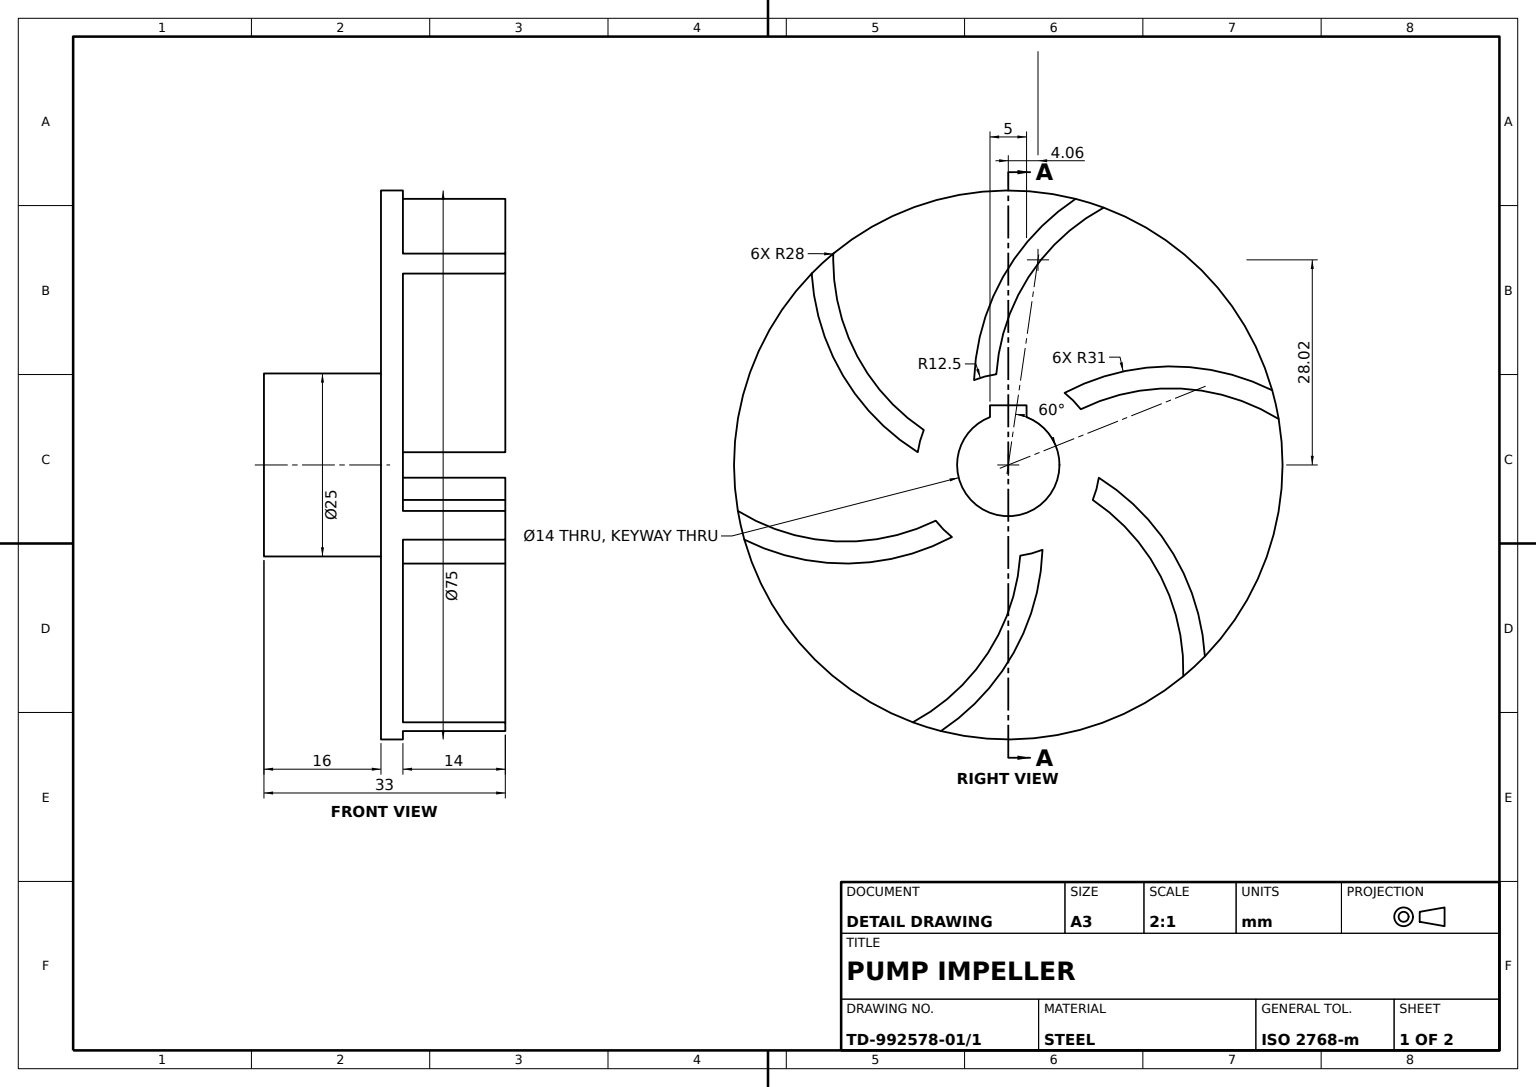
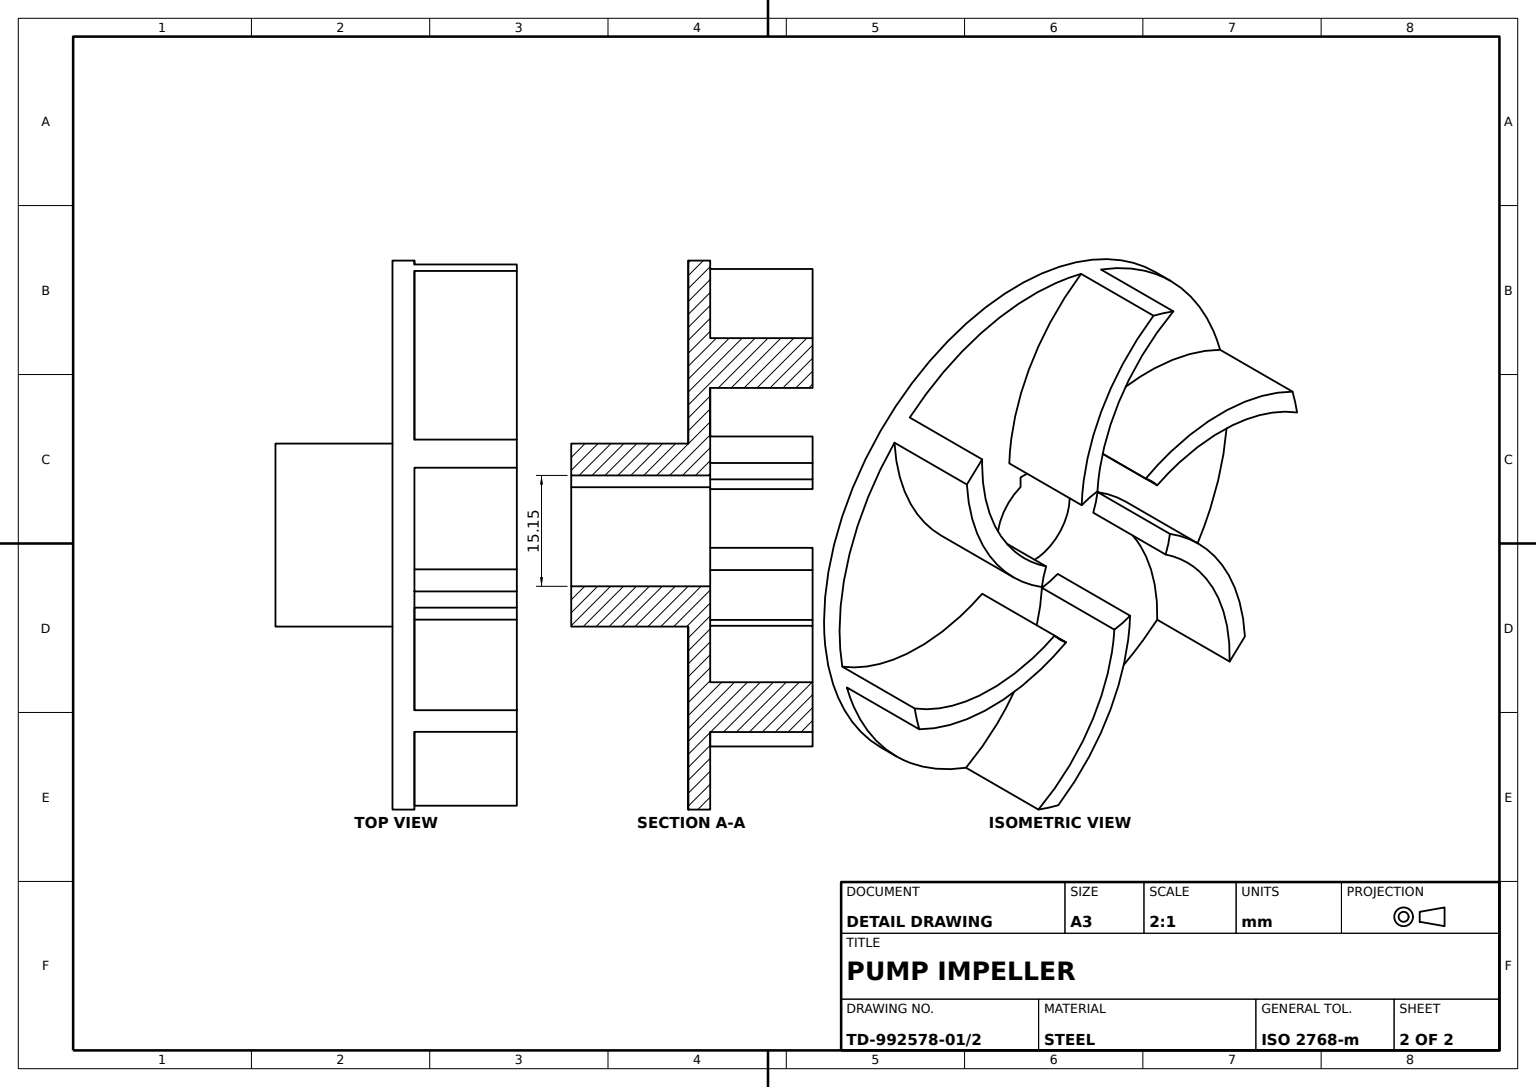
SolidWorks part; units mm, degrees
material "Plain Carbon Steel"
ref_plane "Front Plane" through (0, 0, 0) normal (0, 0, 1) x (1, 0, 0)
ref_plane "Top Plane" through (0, 0, 0) normal (0, 1, 0) x (1, 0, 0)
ref_plane "Right Plane" through (0, 0, 0) normal (1, 0, 0) x (0, 0, -1)
sketch "Hub Disc Profile" plane through (0, 0, 0) normal (0, 0, 1) x (1, 0, 0)
  line L0 (0, 12.5) -> (0, -20.8889) construction
  line L1 (-28, 0) -> (30.1111, 0) construction
  line L2 (0, 12.5) -> (0, 7)
  line L4 (0, 12.5) -> (16, 12.5)
  line L5 (16, 12.5) -> (16, 37.5)
  line L6 (16, 37.5) -> (19, 37.5)
  line L7 (19, 37.5) -> (19, 7)
  line L12 (0, 7) -> (19, 7)
  dimension "D1" = 3
  dimension "D2" = 16
  dimension "D3" = 19
  dimension "D4" = 5.5
  dimension "D5" = 30.5
  dimension "D6" = 37.5
revolve "Hub and Back Disc" add sketch "Hub Disc Profile" angle 360 about L1
sketch "Shaft Bore Profile" plane through (0, 0, 0) normal (-1, 0, 0) x (0, 0, 1)
  line L0 (0, 0) -> (0, 24.4798) construction
  line L2 (-2.5, 8.15) -> (2.5, 8.15)
  line L3 (-2.5, 8.15) -> (-2.5, 5.85)
  line L4 (-2.5, 5.85) -> (2.5, 5.85)
  line L5 (2.5, 8.15) -> (2.5, 5.85)
  line L6 (-2.5, 8.15) -> (2.5, 5.85) construction
  line L7 (-2.5, 5.85) -> (2.5, 8.15) construction
  circle A0 centre (0, 0) radius 7 construction
  point P3 (0, 7)
  dimension "D1" = 5
  dimension "D2" = 8.15
extrude "Shaft Bore" cut sketch "Shaft Bore Profile" against normal blind 30
sketch "Vane Profiles 6x" plane through (19, 0, 0) normal (1, 0, 0) x (0, 0, -1)
  line L0 (-2.5, 6.5383) -> (-2.5, 8.15) construction
  circle A1 centre (0, 0) radius 37.5
  arc A2 (-23.9243, 28.8769) -> (-26.8807, 26.1473) centre (0, 0) ccw
  arc A7 (-11.5505, 4.7787) -> (-12.3782, 1.7404) centre (0, 0) ccw
  arc A8 (-23.9243, 28.8769) -> (-11.5505, 4.7787) centre (4.0626, 28.0216) ccw
  arc A9 (-26.8807, 26.1473) -> (-12.3782, 1.7404) centre (4.0626, 28.0216) ccw
  arc A10 (13.046, 35.1575) -> (-1.6368, 12.3924) centre (26.2987, 10.4925) ccw
  arc A11 (9.2038, 36.353) -> (-4.6819, 11.5901) centre (26.2987, 10.4925) ccw
  arc A12 (-1.6368, 12.3924) -> (-4.6819, 11.5901) centre (0, 0) ccw
  arc A13 (36.9703, 6.2806) -> (9.9137, 7.6137) centre (22.2361, -17.5291) ccw
  arc A14 (36.0845, 10.2057) -> (7.6964, 9.8497) centre (22.2361, -17.5291) ccw
  arc A15 (9.9137, 7.6137) -> (7.6964, 9.8497) centre (0, 0) ccw
  arc A16 (23.9243, -28.8769) -> (11.5505, -4.7787) centre (-4.0626, -28.0216) ccw
  arc A17 (26.8807, -26.1473) -> (12.3782, -1.7404) centre (-4.0626, -28.0216) ccw
  arc A18 (11.5505, -4.7787) -> (12.3782, -1.7404) centre (0, 0) ccw
  arc A19 (-13.046, -35.1575) -> (1.6368, -12.3924) centre (-26.2987, -10.4925) ccw
  arc A20 (-9.2038, -36.353) -> (4.6819, -11.5901) centre (-26.2987, -10.4925) ccw
  arc A21 (1.6368, -12.3924) -> (4.6819, -11.5901) centre (0, 0) ccw
  arc A22 (-36.9703, -6.2806) -> (-9.9137, -7.6137) centre (-22.2361, 17.5291) ccw
  arc A23 (-36.0845, -10.2057) -> (-7.6964, -9.8497) centre (-22.2361, 17.5291) ccw
  arc A24 (-9.9137, -7.6137) -> (-7.6964, -9.8497) centre (0, 0) ccw
  arc A29 (13.046, 35.1575) -> (9.2038, 36.353) centre (0, 0) ccw
  arc A30 (36.9703, 6.2806) -> (36.0845, 10.2057) centre (0, 0) ccw
  arc A31 (23.9243, -28.8769) -> (26.8807, -26.1473) centre (0, 0) ccw
  arc A32 (-13.046, -35.1575) -> (-9.2038, -36.353) centre (0, 0) ccw
  arc A33 (-36.9703, -6.2806) -> (-36.0845, -10.2057) centre (0, 0) ccw
  point P38 (0, 0)
  point P48 (0, 0)
  circle M6 centre (0, 0) radius 37.5
  dimension "D2" = 12.5
  dimension "D3" = 6
  dimension "D4" = 28
  dimension "D5" = 31
  dimension "D6" = 0.8632
  dimension "D7" = 6.5626
  dimension "D1" = 0
extrude "Vanes 6x" add sketch "Vane Profiles 6x" along normal blind 14 contours A24 A22 A23 M6 | A21 A19 A20 M6 | A18 A16 A17 M6 | A12 A10 A11 M6 | A8 A7 A9 A2 | A14 A15 A13 A30
